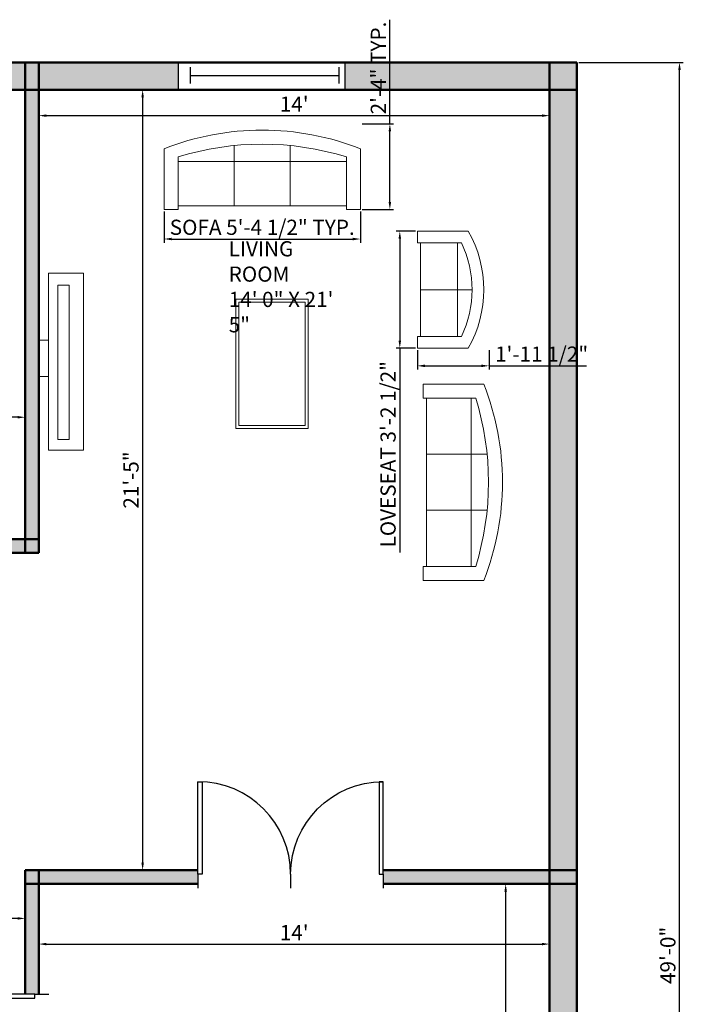
# Model space of a CAD drawing. Units: millimetres. Extents: x 3107 to 3757, y 777 to 1464.
# Tile 7 of 7: x 3539 to 3757, y 1140 to 1464. Entities that reach past the tile are written whole.
import ezdxf

# ---------------------------------------------------------------- set-up
doc = ezdxf.new("R2010")
doc.units = ezdxf.units.MM
for name, color, linetype, lineweight in [('A-ANNO-DIMS', 50, 'Continuous', 18), ('A-AREA-IDEN', 160, 'Continuous', 18), ('A-EQPM', 140, 'Continuous', 18), ('A-WALL-PATT', 80, 'Continuous', 13), ('doors', 10, 'Continuous', 25), ('furniture', 140, 'Continuous', 18), ('walls', 80, 'Continuous', 50), ('windows', 30, 'Continuous', 25)]:
    doc.layers.add(name, color=color, linetype=linetype, lineweight=lineweight)
doc.styles.get("Standard").update_dxf_attribs({"font": 'arial.ttf'})
doc.dimstyles.new('ISO-25', dxfattribs={"dimtxt": 5, "dimasz": 2.5, "dimexe": 1.25, "dimexo": 0.625, "dimtad": 1, "dimdec": 0, "dimlunit": 3, "dimtxsty": 'Standard', "dimcen": 2.5, "dimadec": 0, "dimazin": 0, "dimtfac": 1, "dimtdec": 0, "dimtmove": 0, "dimatfit": 3, "dimfxl": 1, "dimarcsym": 0})

# ---------------------------------------------------------------- blocks, each defined once
blk = doc.blocks.new('*U2')
for p, q in [((0, 0), (0, -6)), ((40, 0), (40, -6))]:
    blk.add_line(p, q)
blk.add_lwpolyline([(0, 0), (0, 40), (1.75, 40), (1.75, 0)], close=True)
blk.add_arc((0, 0), 40, 0, 90)
blk = doc.blocks.new('*U4')
for p, q in [((0, 4), (0, 0)), ((36, 4), (36, 0)), ((0, 2), (36, 2))]:
    blk.add_line(p, q)
blk = doc.blocks.new('Sofa - Roundback 7 ft.')
for p, q in [((-12.00002, -32.4421), (-12.00003, -6.5971)), ((11.99997, -32.4421), (11.99998, -6.5971)), ((-36.000027, -34), (-36.000027, -11.4696)), ((35.99998, -34), (35.99998, -11.4696)), ((-35.999844, -13.3819), (35.9998, -13.3819)), ((-36.000027, -32.4421), (35.99998, -32.4421))]:
    blk.add_line(p, q)
for points in [[(-36.000027, -34), (-42.000027, -34), (-42.000027, -8)], [(41.99998, -8), (41.99998, -34), (35.99998, -34)]]:
    blk.add_lwpolyline(points)
for centre, radius, start, end in [((0, -114.25), 114.25, 68.43141, 111.5686), ((-0.00001, -127.1968), 121.1968, 72.72033, 107.2797)]:
    blk.add_arc(centre, radius, start, end)
blk = doc.blocks.new('Sofa - Roundback Loveseat 5 ft.')
for p, q in [((0, -32.44198), (0, -5.99998)), ((-24, -33.99998), (-24, -11.46958)), ((-23.9998, -13.38178), (23.99986, -13.38178)), ((24.00004, -33.99998), (24.00004, -11.46958)), ((-24, -32.44198), (24.00004, -32.44198))]:
    blk.add_line(p, q)
for points in [[(-24, -33.99998), (-30, -33.99998), (-30, -7.99998)], [(30.00004, -7.99998), (30.00004, -33.99998), (24.00004, -33.99998)]]:
    blk.add_lwpolyline(points)
for centre, radius, start, end in [((0, -60.24998), 60.24998, 60.13715, 119.8628), ((0, -61.38438), 55.38444, 64.32083, 115.6792)]:
    blk.add_arc(centre, radius, start, end)
blk = doc.blocks.new('*D20')
at = {"layer": 'A-ANNO-DIMS', "color": 0, "lineweight": -2, "transparency": 16777216}
for p, q in [((3384.47, 1334.22), (3384.47, 1334.85)), ((3537.97, 1333.6), (3386.97, 1333.6)), ((3540.47, 1332.97), (3540.47, 1332.35))]:
    blk.add_line(p, q, dxfattribs=at)
at = {"layer": 'A-ANNO-DIMS', "color": 0, "transparency": 16777216}
for points in [[(3386.97, 1334.01), (3386.97, 1333.18), (3384.47, 1333.6)], [(3537.97, 1334.01), (3537.97, 1333.18), (3540.47, 1333.6)]]:
    blk.add_solid(points, dxfattribs=at)
at = {"layer": 'Defpoints', "color": 0, "transparency": 16777216}
for p in [(3384.47, 1333.6), (3384.47, 1333.6), (3540.47, 1333.6)]:
    blk.add_point(p, dxfattribs=at)
at = {"layer": 'A-ANNO-DIMS', "color": 0, "transparency": 16777216, "insert": (3462.47, 1336.78), "char_height": 5, "attachment_point": 5}
blk.add_mtext("13'", dxfattribs=at)
blk = doc.blocks.new('*D22')
at = {"layer": 'A-ANNO-DIMS', "color": 0, "lineweight": -2, "transparency": 16777216}
for p, q in [((3544.97, 1433.26), (3544.97, 1431.65)), ((3547.47, 1432.9), (3710.47, 1432.9)), ((3712.97, 1433.26), (3712.97, 1431.65))]:
    blk.add_line(p, q, dxfattribs=at)
at = {"layer": 'A-ANNO-DIMS', "color": 0, "transparency": 16777216}
for points in [[(3547.47, 1433.32), (3547.47, 1432.49), (3544.97, 1432.9)], [(3710.47, 1433.32), (3710.47, 1432.49), (3712.97, 1432.9)]]:
    blk.add_solid(points, dxfattribs=at)
at = {"layer": 'Defpoints', "color": 0, "transparency": 16777216}
for p in [(3544.97, 1433.88), (3712.97, 1433.88), (3712.97, 1432.9)]:
    blk.add_point(p, dxfattribs=at)
at = {"layer": 'A-ANNO-DIMS', "color": 0, "transparency": 16777216, "insert": (3628.97, 1436.04), "char_height": 5, "attachment_point": 5}
blk.add_mtext("14'", dxfattribs=at)
blk = doc.blocks.new('*D23')
at = {"layer": 'A-ANNO-DIMS', "color": 0, "lineweight": -2, "transparency": 16777216}
for p, q in [((3569.79, 1441.43), (3580.37, 1441.43)), ((3579.12, 1438.93), (3579.12, 1186.93)), ((3578.06, 1184.43), (3580.37, 1184.43))]:
    blk.add_line(p, q, dxfattribs=at)
at = {"layer": 'A-ANNO-DIMS', "color": 0, "transparency": 16777216}
for points in [[(3578.7, 1438.93), (3579.53, 1438.93), (3579.12, 1441.43)], [(3578.7, 1186.93), (3579.53, 1186.93), (3579.12, 1184.43)]]:
    blk.add_solid(points, dxfattribs=at)
at = {"layer": 'Defpoints', "color": 0, "transparency": 16777216}
for p in [(3569.16, 1441.43), (3577.44, 1184.43), (3579.12, 1184.43)]:
    blk.add_point(p, dxfattribs=at)
at = {"layer": 'A-ANNO-DIMS', "color": 0, "transparency": 16777216, "insert": (3575.94, 1312.93), "char_height": 5, "attachment_point": 5, "rotation": 90}
blk.add_mtext('21\'-5"', dxfattribs=at)
blk = doc.blocks.new('*D41')
at = {"layer": 'A-ANNO-DIMS', "color": 0, "lineweight": -2, "transparency": 16777216}
for p, q in [((3352.47, 1164.68), (3352.47, 1169.84)), ((3537.97, 1168.59), (3354.97, 1168.59)), ((3540.47, 1164.68), (3540.47, 1169.84))]:
    blk.add_line(p, q, dxfattribs=at)
at = {"layer": 'A-ANNO-DIMS', "color": 0, "transparency": 16777216}
for points in [[(3354.97, 1169), (3354.97, 1168.17), (3352.47, 1168.59)], [(3537.97, 1169), (3537.97, 1168.17), (3540.47, 1168.59)]]:
    blk.add_solid(points, dxfattribs=at)
at = {"layer": 'Defpoints', "color": 0, "transparency": 16777216}
for p in [(3352.47, 1168.59), (3352.47, 1164.06), (3540.47, 1164.06)]:
    blk.add_point(p, dxfattribs=at)
at = {"layer": 'A-ANNO-DIMS', "color": 0, "transparency": 16777216, "insert": (3446.47, 1171.76), "char_height": 5, "attachment_point": 5}
blk.add_mtext('15\'-8"', dxfattribs=at)
blk = doc.blocks.new('*D42')
at = {"layer": 'A-ANNO-DIMS', "color": 0, "lineweight": -2, "transparency": 16777216}
for p, q in [((3544.97, 1163.63), (3544.97, 1158.9)), ((3712.97, 1163.63), (3712.97, 1158.9)), ((3547.47, 1160.15), (3710.47, 1160.15))]:
    blk.add_line(p, q, dxfattribs=at)
at = {"layer": 'A-ANNO-DIMS', "color": 0, "transparency": 16777216}
for points in [[(3547.47, 1160.56), (3547.47, 1159.73), (3544.97, 1160.15)], [(3710.47, 1160.56), (3710.47, 1159.73), (3712.97, 1160.15)]]:
    blk.add_solid(points, dxfattribs=at)
at = {"layer": 'Defpoints', "color": 0, "transparency": 16777216}
for p in [(3544.97, 1164.25), (3712.97, 1164.25), (3712.97, 1160.15)]:
    blk.add_point(p, dxfattribs=at)
at = {"layer": 'A-ANNO-DIMS', "color": 0, "transparency": 16777216, "insert": (3628.97, 1163.28), "char_height": 5, "attachment_point": 5}
blk.add_mtext("14'", dxfattribs=at)
blk = doc.blocks.new('*D43')
at = {"layer": 'A-ANNO-DIMS', "color": 0, "lineweight": -2, "transparency": 16777216}
for p, q in [((3694.45, 1179.93), (3699.81, 1179.93)), ((3698.56, 1177.43), (3698.56, 873.93)), ((3687.78, 871.43), (3699.81, 871.43))]:
    blk.add_line(p, q, dxfattribs=at)
at = {"layer": 'A-ANNO-DIMS', "color": 0, "transparency": 16777216}
for points in [[(3698.14, 1177.43), (3698.97, 1177.43), (3698.56, 1179.93)], [(3698.14, 873.93), (3698.97, 873.93), (3698.56, 871.43)]]:
    blk.add_solid(points, dxfattribs=at)
at = {"layer": 'Defpoints', "color": 0, "transparency": 16777216}
for p in [(3693.82, 1179.93), (3687.15, 871.43), (3698.56, 871.43)]:
    blk.add_point(p, dxfattribs=at)
at = {"layer": 'A-ANNO-DIMS', "color": 0, "transparency": 16777216, "insert": (3695.38, 1025.68), "char_height": 5, "attachment_point": 5, "rotation": 90}
blk.add_mtext('25\'-9"', dxfattribs=at)
blk = doc.blocks.new('*D53')
at = {"layer": 'A-ANNO-DIMS', "color": 0, "lineweight": -2, "transparency": 16777216}
for p, q in [((3586.15, 1401.35), (3586.15, 1391.03)), ((3650.77, 1401.35), (3650.77, 1391.03)), ((3588.65, 1392.28), (3648.27, 1392.28))]:
    blk.add_line(p, q, dxfattribs=at)
at = {"layer": 'A-ANNO-DIMS', "color": 0, "transparency": 16777216}
for points in [[(3588.65, 1392.7), (3588.65, 1391.86), (3586.15, 1392.28)], [(3648.27, 1392.7), (3648.27, 1391.86), (3650.77, 1392.28)]]:
    blk.add_solid(points, dxfattribs=at)
at = {"layer": 'Defpoints', "color": 0, "transparency": 16777216}
for p in [(3586.15, 1401.97), (3650.77, 1401.97), (3650.77, 1392.28)]:
    blk.add_point(p, dxfattribs=at)
at = {"layer": 'A-ANNO-DIMS', "color": 0, "transparency": 16777216, "insert": (3618.46, 1395.49), "char_height": 5, "attachment_point": 5}
blk.add_mtext('SOFA 5\'-4 1/2" TYP.', dxfattribs=at)
blk = doc.blocks.new('*D54')
at = {"layer": 'A-ANNO-DIMS', "color": 0, "lineweight": -2, "transparency": 16777216}
for p, q in [((3660.46, 1430.18), (3660.46, 1464.49)), ((3651.39, 1430.18), (3661.71, 1430.18)), ((3660.46, 1404.47), (3660.46, 1427.68)), ((3651.39, 1401.97), (3661.71, 1401.97))]:
    blk.add_line(p, q, dxfattribs=at)
at = {"layer": 'A-ANNO-DIMS', "color": 0, "transparency": 16777216}
for points in [[(3660.04, 1427.68), (3660.88, 1427.68), (3660.46, 1430.18)], [(3660.04, 1404.47), (3660.88, 1404.47), (3660.46, 1401.97)]]:
    blk.add_solid(points, dxfattribs=at)
at = {"layer": 'Defpoints', "color": 0, "transparency": 16777216}
for p in [(3650.77, 1430.18), (3660.46, 1430.18), (3650.77, 1401.97)]:
    blk.add_point(p, dxfattribs=at)
at = {"layer": 'A-ANNO-DIMS', "color": 0, "transparency": 16777216, "insert": (3657.32, 1448.58), "char_height": 5, "attachment_point": 5, "rotation": 90}
blk.add_mtext('2\'-4" TYP.', dxfattribs=at)
blk = doc.blocks.new('*D57')
at = {"layer": 'A-ANNO-DIMS', "color": 0, "lineweight": -2, "transparency": 16777216}
for p, q in [((3668.89, 1394.89), (3662.48, 1394.89)), ((3663.73, 1392.39), (3663.73, 1358.81)), ((3668.89, 1356.31), (3662.48, 1356.31)), ((3663.73, 1356.31), (3663.73, 1289.02))]:
    blk.add_line(p, q, dxfattribs=at)
at = {"layer": 'A-ANNO-DIMS', "color": 0, "transparency": 16777216}
for points in [[(3663.31, 1392.39), (3664.15, 1392.39), (3663.73, 1394.89)], [(3663.31, 1358.81), (3664.15, 1358.81), (3663.73, 1356.31)]]:
    blk.add_solid(points, dxfattribs=at)
at = {"layer": 'Defpoints', "color": 0, "transparency": 16777216}
for p in [(3669.52, 1394.89), (3663.73, 1356.31), (3669.52, 1356.31)]:
    blk.add_point(p, dxfattribs=at)
at = {"layer": 'A-ANNO-DIMS', "color": 0, "transparency": 16777216, "insert": (3660.52, 1321.42), "char_height": 5, "attachment_point": 5, "rotation": 90}
blk.add_mtext('LOVESEAT 3\'-2 1/2"', dxfattribs=at)
blk = doc.blocks.new('*D58')
at = {"layer": 'A-ANNO-DIMS', "color": 0, "lineweight": -2, "transparency": 16777216}
for p, q in [((3669.52, 1355.69), (3669.52, 1349.27)), ((3693.09, 1355.69), (3693.09, 1349.27)), ((3672.02, 1350.52), (3690.59, 1350.52)), ((3693.09, 1350.52), (3725.19, 1350.52))]:
    blk.add_line(p, q, dxfattribs=at)
at = {"layer": 'A-ANNO-DIMS', "color": 0, "transparency": 16777216}
for points in [[(3672.02, 1350.94), (3672.02, 1350.11), (3669.52, 1350.52)], [(3690.59, 1350.94), (3690.59, 1350.11), (3693.09, 1350.52)]]:
    blk.add_solid(points, dxfattribs=at)
at = {"layer": 'Defpoints', "color": 0, "transparency": 16777216}
for p in [(3669.52, 1356.31), (3693.09, 1356.31), (3693.09, 1350.52)]:
    blk.add_point(p, dxfattribs=at)
at = {"layer": 'A-ANNO-DIMS', "color": 0, "transparency": 16777216, "insert": (3710.39, 1353.74), "char_height": 5, "attachment_point": 5}
blk.add_mtext('1\'-11 1/2"', dxfattribs=at)
blk = doc.blocks.new('*D70')
at = {"layer": 'A-ANNO-DIMS', "color": 0, "lineweight": -2, "transparency": 16777216}
for p, q in [((3722.59, 1450.43), (3757.01, 1450.43)), ((3755.76, 864.93), (3755.76, 1447.93)), ((3722.59, 862.43), (3757.01, 862.43))]:
    blk.add_line(p, q, dxfattribs=at)
at = {"layer": 'A-ANNO-DIMS', "color": 0, "transparency": 16777216}
for points in [[(3755.34, 1447.93), (3756.17, 1447.93), (3755.76, 1450.43)], [(3755.34, 864.93), (3756.17, 864.93), (3755.76, 862.43)]]:
    blk.add_solid(points, dxfattribs=at)
at = {"layer": 'Defpoints', "color": 0, "transparency": 16777216}
for p in [(3721.97, 1450.43), (3755.76, 1450.43), (3721.97, 862.43)]:
    blk.add_point(p, dxfattribs=at)
at = {"layer": 'A-ANNO-DIMS', "color": 0, "transparency": 16777216, "insert": (3752.58, 1156.43), "char_height": 5, "attachment_point": 5, "rotation": 90}
blk.add_mtext('49\'-0"', dxfattribs=at)

msp = doc.modelspace()

# ---------------------------------------------------------------- hatches: boundary and pattern name
at = {"layer": 'A-WALL-PATT'}
h = msp.add_hatch(color=256, dxfattribs=at)
h.dxf.hatch_style = 1
h.paths.add_polyline_path([(3119.47, 1087.39), (3110.47, 1087.39), (3110.47, 1027.93), (3119.47, 1027.93)])
h.paths.add_polyline_path([(3119.47, 1027.93), (3110.47, 1027.93), (3110.47, 1023.43), (3119.47, 1023.43)])
h.paths.add_polyline_path([(3267.47, 1027.93), (3119.47, 1027.93), (3119.47, 1023.43), (3267.47, 1023.43)])
h.paths.add_polyline_path([(3119.47, 1023.43), (3110.47, 1023.43), (3110.47, 979.44), (3119.47, 979.44)])
h.paths.add_polyline_path([(3299.97, 1179.93), (3295.47, 1179.93), (3295.47, 1027.93), (3299.97, 1027.93)])
h.paths.add_polyline_path([(3295.47, 1027.93), (3271.97, 1027.93), (3271.97, 1023.43), (3295.47, 1023.43)])
h.paths.add_polyline_path([(3271.97, 1027.93), (3267.47, 1027.93), (3267.47, 1023.43), (3271.97, 1023.43)])
h.paths.add_polyline_path([(3299.97, 1027.93), (3295.47, 1027.93), (3295.47, 1023.43), (3299.97, 1023.43)])
h.paths.add_polyline_path([(3299.97, 1184.43), (3295.47, 1184.43), (3295.47, 1179.93), (3299.97, 1179.93)])
h.paths.add_polyline_path([(3295.47, 1184.43), (3288.38, 1184.43), (3288.38, 1182.47), (3288.38, 1179.93), (3295.47, 1179.93)])
h.paths.add_polyline_path([(3352.47, 1179.93), (3347.97, 1179.93), (3347.97, 1027.93), (3352.47, 1027.93)])
h.paths.add_polyline_path([(3352.47, 1184.43), (3347.97, 1184.43), (3347.97, 1179.93), (3352.47, 1179.93)])
h.paths.add_polyline_path([(3464.47, 1184.43), (3352.47, 1184.43), (3352.47, 1179.93), (3464.47, 1179.93)])
h.paths.add_polyline_path([(3468.97, 1288.93), (3464.47, 1288.93), (3464.47, 1184.43), (3468.97, 1184.43)])
h.paths.add_polyline_path([(3468.97, 1184.43), (3464.47, 1184.43), (3464.47, 1179.93), (3468.97, 1179.93)])
h.paths.add_polyline_path([(3195.97, 1248.43), (3191.47, 1248.43), (3191.47, 1184.43), (3195.97, 1184.43)])
h.paths.add_polyline_path([(3195.97, 1184.43), (3191.47, 1184.43), (3191.47, 1179.93), (3195.97, 1179.93)])
h.paths.add_polyline_path([(3191.47, 1184.43), (3183.28, 1184.43), (3183.28, 1181.58), (3183.28, 1179.93), (3191.47, 1179.93)])
h.paths.add_polyline_path([(3243.97, 1184.43), (3195.97, 1184.43), (3195.97, 1179.93), (3243.97, 1179.93)])
h.paths.add_polyline_path([(3257.91, 1182.47), (3257.91, 1184.43), (3248.47, 1184.43), (3248.47, 1179.93), (3258.02, 1179.93, -0.020891)])
h.paths.add_polyline_path([(3248.47, 1184.43), (3243.97, 1184.43), (3243.97, 1179.93), (3248.47, 1179.93)])
h.paths.add_polyline_path([(3248.47, 1189.24), (3247.51, 1189.24), (3243.97, 1189.24), (3243.97, 1184.43), (3248.47, 1184.43)])
h.paths.add_polyline_path([(3166.87, 1184.43), (3119.47, 1184.43), (3119.47, 1179.93), (3166.63, 1179.93), (3166.63, 1181.58, -0.042981)])
h.paths.add_polyline_path([(3119.47, 1184.43), (3110.47, 1184.43), (3110.47, 1179.93), (3119.47, 1179.93)])
h.paths.add_polyline_path([(3119.47, 1248.43), (3110.47, 1248.43), (3110.47, 1184.43), (3119.47, 1184.43)])
h.paths.add_polyline_path([(3119.47, 1179.93), (3110.47, 1179.93), (3110.47, 1140.65), (3119.47, 1140.65)])
h.paths.add_polyline_path([(3119.47, 1288.93), (3110.47, 1288.93), (3110.47, 1252.93), (3119.47, 1252.93)])
h.paths.add_polyline_path([(3119.47, 1252.93), (3110.47, 1252.93), (3110.47, 1248.43), (3119.47, 1248.43)])
h.paths.add_polyline_path([(3191.47, 1252.93), (3119.47, 1252.93), (3119.47, 1248.43), (3191.47, 1248.43)])
h.paths.add_polyline_path([(3195.97, 1288.93), (3191.47, 1288.93), (3191.47, 1252.93), (3195.97, 1252.93)])
h.paths.add_polyline_path([(3195.97, 1252.93), (3191.47, 1252.93), (3191.47, 1248.43), (3195.97, 1248.43)])
h.paths.add_polyline_path([(3248.47, 1293.43), (3243.97, 1293.43), (3243.97, 1288.93), (3248.47, 1288.93)])
h.paths.add_polyline_path([(3243.97, 1293.43), (3195.97, 1293.43), (3195.97, 1288.93), (3243.97, 1288.93)])
h.paths.add_polyline_path([(3303.47, 1293.43), (3248.47, 1293.43), (3248.47, 1288.93), (3303.47, 1288.93)])
h.paths.add_polyline_path([(3248.47, 1288.93), (3243.97, 1288.93), (3243.97, 1205.51, -0.053712), (3247.51, 1205.89), (3248.47, 1205.89)])
h.paths.add_polyline_path([(3191.47, 1293.43), (3119.47, 1293.43), (3119.47, 1288.93), (3191.47, 1288.93)])
h.paths.add_polyline_path([(3119.47, 1293.43), (3110.47, 1293.43), (3110.47, 1288.93), (3119.47, 1288.93)])
h.paths.add_polyline_path([(3119.47, 1322.96, -0.065064), (3111.64, 1321.93), (3110.47, 1321.93), (3110.47, 1293.43), (3119.47, 1293.43)])
h.paths.add_polyline_path([(3195.97, 1293.43), (3191.47, 1293.43), (3191.47, 1288.93), (3195.97, 1288.93)])
h.paths.add_polyline_path([(3119.47, 1450.43), (3110.47, 1450.43), (3110.47, 1441.43), (3119.47, 1441.43)])
h.paths.add_polyline_path([(3119.47, 1441.43), (3110.47, 1441.43), (3110.47, 1352.4), (3111.64, 1352.4), (3119.47, 1352.4)])
h.paths.add_polyline_path([(3176.58, 1450.43), (3119.47, 1450.43), (3119.47, 1441.43), (3176.58, 1441.43)])
h.paths.add_polyline_path([(3323.19, 1450.43), (3307.97, 1450.43), (3307.97, 1441.43), (3323.19, 1441.43)])
h.paths.add_polyline_path([(3307.97, 1450.43), (3303.47, 1450.43), (3303.47, 1441.43), (3307.97, 1441.43)])
h.paths.add_polyline_path([(3303.47, 1450.43), (3229.4, 1450.43), (3229.4, 1441.43), (3303.47, 1441.43)])
h.paths.add_polyline_path([(3307.97, 1441.43), (3303.47, 1441.43), (3303.47, 1363.43), (3307.97, 1363.43)])
h.paths.add_polyline_path([(3307.97, 1363.43), (3303.47, 1363.43), (3303.47, 1358.93), (3307.97, 1358.93)])
h.paths.add_polyline_path([(3307.97, 1358.93), (3303.47, 1358.93), (3303.47, 1342.3), (3305.5, 1342.3, -0.037178), (3307.97, 1342.12)])
h.paths.add_polyline_path([(3379.97, 1363.43), (3307.97, 1363.43), (3307.97, 1358.93), (3379.97, 1358.93)])
h.paths.add_polyline_path([(3384.47, 1393.61), (3383.04, 1393.61), (3379.97, 1393.61), (3379.97, 1363.43), (3384.47, 1363.43)])
h.paths.add_polyline_path([(3384.47, 1363.43), (3379.97, 1363.43), (3379.97, 1358.93), (3384.47, 1358.93)])
h.paths.add_polyline_path([(3384.47, 1358.93), (3379.97, 1358.93), (3379.97, 1293.43), (3384.47, 1293.43)])
h.paths.add_polyline_path([(3384.47, 1441.43), (3379.97, 1441.43), (3379.97, 1409.98, -0.046389), (3383.04, 1410.27), (3384.47, 1410.27)])
h.paths.add_polyline_path([(3384.47, 1450.43), (3379.97, 1450.43), (3379.97, 1441.43), (3384.47, 1441.43)])
h.paths.add_polyline_path([(3379.97, 1450.43), (3357.18, 1450.43), (3357.18, 1441.43), (3379.97, 1441.43)])
h.paths.add_polyline_path([(3432.79, 1450.43), (3384.47, 1450.43), (3384.47, 1441.43), (3432.79, 1441.43)])
h.paths.add_polyline_path([(3540.47, 1450.43), (3484.18, 1450.43), (3484.18, 1441.43), (3540.47, 1441.43)])
h.paths.add_polyline_path([(3544.97, 1450.43), (3540.47, 1450.43), (3540.47, 1441.43), (3544.97, 1441.43)])
h.paths.add_polyline_path([(3544.97, 1441.43), (3540.47, 1441.43), (3540.47, 1293.43), (3544.97, 1293.43)])
h.paths.add_polyline_path([(3590.83, 1450.43), (3544.97, 1450.43), (3544.97, 1441.43), (3590.83, 1441.43)])
h.paths.add_polyline_path([(3712.97, 1450.43), (3645.62, 1450.43), (3645.62, 1441.43), (3712.97, 1441.43)])
h.paths.add_polyline_path([(3721.97, 1441.43), (3712.97, 1441.43), (3712.97, 1288.93), (3712.97, 1184.43), (3721.97, 1184.43), (3721.97, 1288.93)])
h.paths.add_polyline_path([(3721.97, 1450.43), (3712.97, 1450.43), (3712.97, 1441.43), (3721.97, 1441.43)])
h.paths.add_polyline_path([(3712.97, 1184.43), (3658.24, 1184.43), (3658.24, 1183.15), (3658.24, 1179.93), (3712.97, 1179.93)])
h.paths.add_polyline_path([(3721.97, 1184.43), (3712.97, 1184.43), (3712.97, 1179.93), (3721.97, 1179.93)])
h.paths.add_polyline_path([(3597.32, 1183.15), (3597.32, 1184.43), (3544.97, 1184.43), (3544.97, 1179.93), (3597.32, 1179.93)])
h.paths.add_polyline_path([(3544.97, 1184.43), (3540.47, 1184.43), (3540.47, 1179.93), (3544.97, 1179.93)])
h.paths.add_polyline_path([(3544.97, 1179.93), (3540.47, 1179.93), (3540.47, 1143.69), (3543.65, 1143.69), (3544.97, 1143.69)])
h.paths.add_polyline_path([(3721.97, 1179.93), (3712.97, 1179.93), (3712.97, 1006.22), (3712.97, 871.43), (3721.97, 871.43), (3721.97, 1006.22)])
h.paths.add_polyline_path([(3468.97, 1293.43), (3464.47, 1293.43), (3464.47, 1288.93), (3468.97, 1288.93)])
h.paths.add_polyline_path([(3540.47, 1293.43), (3468.97, 1293.43), (3468.97, 1288.93), (3540.47, 1288.93)])
h.paths.add_polyline_path([(3544.97, 1293.43), (3540.47, 1293.43), (3540.47, 1288.93), (3544.97, 1288.93)])
h.paths.add_polyline_path([(3464.47, 1293.43), (3417.83, 1293.43, -0.015057), (3417.88, 1291.6), (3417.88, 1288.93), (3464.47, 1288.93)])
h.paths.add_polyline_path([(3379.97, 1293.43), (3307.97, 1293.43), (3307.97, 1288.93), (3379.97, 1288.93)])
h.paths.add_polyline_path([(3307.97, 1325.65), (3305.5, 1325.65), (3303.47, 1325.65), (3303.47, 1293.43), (3307.97, 1293.43)])
h.paths.add_polyline_path([(3307.97, 1293.43), (3303.47, 1293.43), (3303.47, 1288.93), (3307.97, 1288.93)])
h.paths.add_polyline_path([(3384.47, 1293.43), (3379.97, 1293.43), (3379.97, 1288.93), (3384.47, 1288.93)])
h.paths.add_polyline_path([(3387.42, 1291.6), (3387.42, 1293.43), (3384.47, 1293.43), (3384.47, 1288.93), (3387.42, 1288.93)])
h.paths.add_polyline_path([(3119.47, 927.28), (3110.47, 927.28), (3110.47, 871.43), (3119.47, 871.43)])
h.paths.add_polyline_path([(3119.47, 871.43), (3110.47, 871.43), (3110.47, 862.43), (3119.47, 862.43)])
h.paths.add_polyline_path([(3267.47, 871.43), (3119.47, 871.43), (3119.47, 862.43), (3267.47, 862.43)])
h.paths.add_polyline_path([(3271.97, 971.43), (3267.47, 971.43), (3267.47, 871.43), (3271.97, 871.43)])
h.paths.add_polyline_path([(3271.97, 871.43), (3267.47, 871.43), (3267.47, 862.43), (3271.97, 862.43)])
h.paths.add_polyline_path([(3287.13, 871.43), (3271.97, 871.43), (3271.97, 862.43), (3287.13, 862.43)])
h.paths.add_polyline_path([(3347.97, 871.43), (3318.96, 871.43), (3318.96, 862.43), (3347.97, 862.43)])
h.paths.add_polyline_path([(3352.47, 971.43), (3347.97, 971.43), (3347.97, 871.43), (3352.47, 871.43)])
h.paths.add_polyline_path([(3352.47, 871.43), (3347.97, 871.43), (3347.97, 862.43), (3352.47, 862.43)])
h.paths.add_polyline_path([(3375.96, 871.43), (3352.47, 871.43), (3352.47, 862.43), (3375.96, 862.43)])
h.paths.add_polyline_path([(3352.47, 975.93), (3347.97, 975.93), (3347.97, 971.43), (3352.47, 971.43)])
h.paths.add_polyline_path([(3352.47, 986.27, -0.01722), (3350.37, 986.2), (3347.97, 986.2), (3347.97, 975.93), (3352.47, 975.93)])
h.paths.add_polyline_path([(3347.97, 975.93), (3292.38, 975.93), (3292.38, 973.47, -0.030785), (3292.25, 971.43), (3347.97, 971.43)])
h.paths.add_polyline_path([(3271.97, 985.98), (3269.95, 985.98), (3267.47, 985.98), (3267.47, 975.93), (3271.97, 975.93)])
h.paths.add_polyline_path([(3271.97, 975.93), (3267.47, 975.93), (3267.47, 971.43), (3271.97, 971.43)])
h.paths.add_polyline_path([(3275.72, 975.93), (3271.97, 975.93), (3271.97, 971.43), (3275.72, 971.43), (3275.72, 973.47)])
h.paths.add_polyline_path([(3271.97, 1023.43), (3267.47, 1023.43), (3267.47, 1016.34, -0.020418), (3269.95, 1016.44), (3271.97, 1016.44)])
h.paths.add_polyline_path([(3352.47, 1023.43), (3347.97, 1023.43), (3347.97, 1016.67), (3350.37, 1016.67), (3352.47, 1016.67)])
h.paths.add_polyline_path([(3352.47, 1027.93), (3347.97, 1027.93), (3347.97, 1023.43), (3352.47, 1023.43)])
h.paths.add_polyline_path([(3476.47, 1027.93), (3352.47, 1027.93), (3352.47, 1023.43), (3476.47, 1023.43)])
h.paths.add_polyline_path([(3540.47, 1027.93), (3480.97, 1027.93), (3480.97, 1023.43), (3540.47, 1023.43)])
h.paths.add_polyline_path([(3480.97, 1027.93), (3476.47, 1027.93), (3476.47, 1023.43), (3480.97, 1023.43)])
h.paths.add_polyline_path([(3480.97, 1023.43), (3476.47, 1023.43), (3476.47, 871.43), (3480.97, 871.43)])
h.paths.add_polyline_path([(3476.47, 871.43), (3429.88, 871.43), (3429.88, 862.43), (3476.47, 862.43)])
h.paths.add_polyline_path([(3480.97, 871.43), (3476.47, 871.43), (3476.47, 862.43), (3480.97, 862.43)])
h.paths.add_polyline_path([(3493.81, 871.43), (3480.97, 871.43), (3480.97, 862.43), (3493.81, 862.43)])
h.paths.add_polyline_path([(3712.97, 871.43), (3525.61, 871.43), (3525.61, 862.43), (3712.97, 862.43)])
h.paths.add_polyline_path([(3721.97, 871.43), (3712.97, 871.43), (3712.97, 862.43), (3721.97, 862.43)])

# ---------------------------------------------------------------- linework, layer by layer
at = {"layer": 'A-EQPM'}
for points in [[(3548.09, 1380.99), (3559.71, 1380.99), (3559.71, 1322.75), (3548.09, 1322.75)], [(3551.26, 1377.12), (3554.96, 1377.12), (3554.96, 1326.27), (3551.26, 1326.27)], [(3548.09, 1359.03), (3544.97, 1359.03), (3544.97, 1347), (3548.09, 1347)]]:
    msp.add_lwpolyline(points, close=True, dxfattribs=at)
at = {"layer": 'furniture'}
for points in [[(3609.8, 1372.46), (3633.63, 1372.46), (3633.63, 1329.89), (3609.8, 1329.89)], [(3610.8, 1371.46), (3632.63, 1371.46), (3632.63, 1330.89), (3610.8, 1330.89)]]:
    msp.add_lwpolyline(points, close=True, dxfattribs=at)
at = {"layer": 'walls'}
for p, q in [((3110.47, 1450.43), (3721.97, 1450.43)), ((3540.47, 1450.43), (3540.47, 1288.93)), ((3544.97, 1450.43), (3544.97, 1288.93)), ((3712.97, 1450.43), (3712.97, 1288.93)), ((3721.97, 1450.43), (3721.97, 1288.93)), ((3110.47, 1441.43), (3721.97, 1441.43)), ((3417.83, 1293.43), (3544.97, 1293.43)), ((3417.88, 1288.93), (3544.97, 1288.93)), ((3712.97, 1288.93), (3712.97, 1006.22)), ((3721.97, 1288.93), (3721.97, 1006.22)), ((3540.47, 1184.43), (3540.47, 1143.69)), ((3540.47, 1184.43), (3597.32, 1184.43)), ((3544.97, 1184.43), (3544.97, 1143.69)), ((3627.75, 1184.43), (3627.81, 1184.43)), ((3658.24, 1184.43), (3721.97, 1184.43)), ((3540.47, 1179.93), (3597.32, 1179.93)), ((3658.24, 1179.93), (3721.97, 1179.93))]:
    msp.add_line(p, q, dxfattribs=at)
at = {"layer": 'windows'}
for p, q in [((3590.83, 1450.43), (3590.83, 1441.43)), ((3645.62, 1450.43), (3645.62, 1441.43))]:
    msp.add_line(p, q, dxfattribs=at)

# ---------------------------------------------------------------- block references
at = {"layer": 'doors', "yscale": 0.7615706373352984, "zscale": 0.7615706373352984}
for p, xscale in [((3597.32, 1183.15), 0.7615706373352984), ((3658.24, 1183.15), -0.7615706373352984)]:
    msp.add_blockref('*U2', p, dxfattribs=dict(at, xscale=xscale))
at = {"layer": 'doors', "xscale": -0.7615706373352984, "yscale": 0.7615706373352984, "zscale": 0.7615706373352984, "rotation": 90.00000000000007}
msp.add_blockref('*U2', (3543.65, 1143.69), dxfattribs=at)
at = {"layer": 'furniture', "xscale": 0.7692352467052823, "yscale": 0.7692352467052823, "zscale": 0.7692352467052823}
msp.add_blockref('Sofa - Roundback 7 ft.', (3618.46, 1428.13), dxfattribs=at)
at = {"layer": 'furniture', "rotation": 270}
for name, p, xscale, yscale, zscale in [('Sofa - Roundback Loveseat 5 ft.', (3691.37, 1375.6), 0.642916848691184, 0.642916848691184, 0.642916848691184), ('Sofa - Roundback 7 ft.', (3697.52, 1312.2), 0.7692352467052823, 0.7692352467052823, 0.7692352467052823)]:
    msp.add_blockref(name, p, dxfattribs=dict(at, xscale=xscale, yscale=yscale, zscale=zscale))
at = {"layer": 'windows', "xscale": 1.357941570966636, "yscale": 1.357941570966636, "zscale": 1.357941570966636}
msp.add_blockref('*U4', (3594.79, 1443.44), dxfattribs=at)

# ---------------------------------------------------------------- texts
at = {"layer": 'A-AREA-IDEN', "insert": (3607.43, 1391.56), "char_height": 5, "attachment_point": 1}
msp.add_mtext_dynamic_manual_height_columns('LIVING ROOM \\P14\' 0" X 21\' 5"', width=41.8182, gutter_width=12.5, heights=[0], dxfattribs=at)

# ---------------------------------------------------------------- dimensions: what is measured, and where the dimension line sits
at = {"layer": 'A-ANNO-DIMS'}
for base, p1, p2, angle, text, picture, middle in [((3660.46, 1430.18), (3650.77, 1401.97), (3650.77, 1430.18), 90, '<> TYP.', '*D54', (3657.32, 1448.58)), ((3663.73, 1356.31), (3669.52, 1394.89), (3669.52, 1356.31), 270, 'LOVESEAT <>', '*D57', (3660.52, 1321.42))]:
    dim = msp.add_linear_dim(base=base, p1=p1, p2=p2, angle=angle, text=text, dimstyle='ISO-25', override={"dimdec": 1, "dimlfac": 1, "dimrnd": 0, "dimzin": 1, "dimdsep": 46, "dimlunit": 4, "dimfrac": 2}, dxfattribs=at)
    dim.commit()
    dim.dimension.update_dxf_attribs({"geometry": picture, "text_midpoint": middle})
for base, p1, p2, override, picture, middle in [((3755.76, 1450.43), (3721.97, 862.43), (3721.97, 1450.43), {"dimdec": 1, "dimlfac": 1, "dimrnd": 0, "dimzin": 1, "dimdsep": 46, "dimlunit": 4, "dimfrac": 2}, '*D70', (3752.58, 1156.43)), ((3579.12, 1184.43), (3569.16, 1441.43), (3577.44, 1184.43), {"dimclrd": 0, "dimclre": 0, "dimclrt": 0}, '*D23', (3575.94, 1312.93)), ((3698.55806305, 871.42857409), (3693.82046366, 1179.92857409), (3687.15261964, 871.42857409), {"dimclrd": 0, "dimclre": 0, "dimclrt": 0}, '*D43', (3695.38019811, 1025.67857409))]:
    dim = msp.add_linear_dim(base=base, p1=p1, p2=p2, angle=90, dimstyle='ISO-25', override=override, dxfattribs=at)
    dim.commit()
    dim.dimension.update_dxf_attribs({"geometry": picture, "text_midpoint": middle})
for base, p1, p2, override, picture, middle in [((3712.97, 1432.9), (3544.97, 1433.88), (3712.97, 1433.88), {"dimclrd": 0, "dimclre": 0, "dimclrt": 0}, '*D22', (3628.97, 1436.04)), ((3693.09, 1350.52), (3669.52, 1356.31), (3693.09, 1356.31), {"dimdec": 1, "dimlfac": 1, "dimrnd": 0, "dimzin": 1, "dimdsep": 46, "dimlunit": 4, "dimfrac": 2}, '*D58', (3710.39, 1353.74)), ((3384.47, 1333.6), (3540.47, 1333.6), (3384.47, 1333.6), {"dimclrd": 0, "dimclre": 0, "dimclrt": 0}, '*D20', (3462.47, 1336.78)), ((3352.47, 1168.59), (3540.47, 1164.06), (3352.47, 1164.06), {"dimclrd": 0, "dimclre": 0, "dimclrt": 0}, '*D41', (3446.47, 1171.76)), ((3712.97, 1160.15), (3544.97, 1164.25), (3712.97, 1164.25), {"dimclrd": 0, "dimclre": 0, "dimclrt": 0}, '*D42', (3628.97, 1163.28))]:
    dim = msp.add_linear_dim(base=base, p1=p1, p2=p2, dimstyle='ISO-25', override=override, dxfattribs=at)
    dim.commit()
    dim.dimension.update_dxf_attribs({"geometry": picture, "text_midpoint": middle})
dim = msp.add_linear_dim(base=(3650.77, 1392.28), p1=(3586.15, 1401.97), p2=(3650.77, 1401.97), text='SOFA <> TYP.', dimstyle='ISO-25', override={"dimdec": 1, "dimlfac": 1, "dimrnd": 0, "dimzin": 1, "dimdsep": 46, "dimlunit": 4, "dimfrac": 2}, dxfattribs=at)
dim.commit()
dim.dimension.update_dxf_attribs({"geometry": '*D53', "text_midpoint": (3618.46, 1395.49)})

doc.saveas('drawing.dxf')
